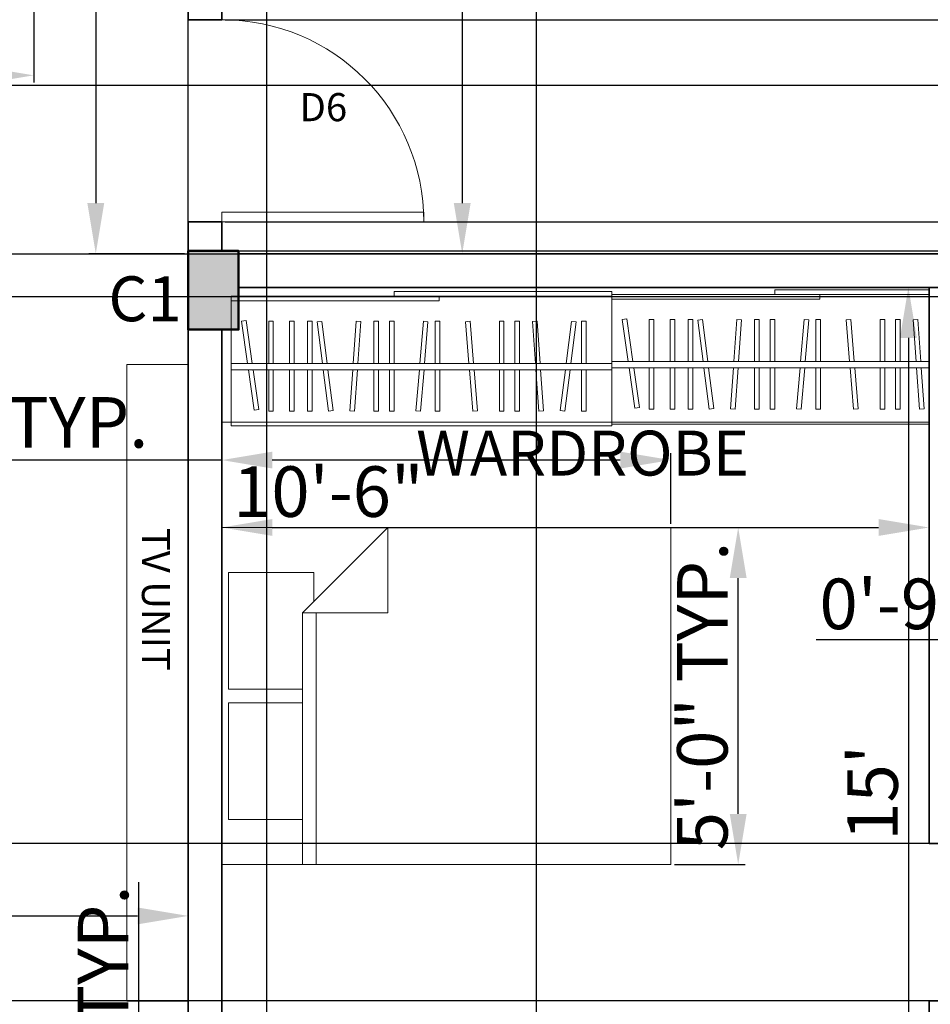
# Model space of a CAD drawing. Units: inches. Extents: x 2621 to 6190, y 513 to 1320.
# Tile 8 of 11: x 2997 to 3160, y 763 to 939. Entities that reach past the tile are written whole.
import ezdxf

# ---------------------------------------------------------------- set-up
doc = ezdxf.new("R2010")
doc.units = ezdxf.units.IN
for name, color, linetype, lineweight in [('A-ANNO-DIMS', 5, 'Continuous', 18), ('A-ANNO-TEXT', 7, 'Continuous', 18), ('A-FLOR-CASE', 30, 'Continuous', 18), ('A-WALL', 7, 'Continuous', 35), ('columns', 2, 'Continuous', 50), ('door', 1, 'Continuous', 18), ('furniture', 30, 'Continuous', 18), ('S-COLS-IDEN', 2, 'Continuous', 25), ('S-COLS-PATT', 2, 'Continuous', 13)]:
    doc.layers.add(name, color=color, linetype=linetype, lineweight=lineweight)
doc.styles.get("Standard").update_dxf_attribs({"font": 'arial.ttf'})
doc.dimstyles.new('ISO-25', dxfattribs={"dimtxt": 9, "dimasz": 9, "dimexe": 1.25, "dimexo": 0.625, "dimtad": 1, "dimlunit": 3, "dimtxsty": 'Standard', "dimcen": 2.5, "dimadec": 0, "dimazin": 0, "dimtfac": 1, "dimtmove": 0, "dimatfit": 3, "dimfxl": 1, "dimarcsym": 0})

# ---------------------------------------------------------------- blocks, each defined once
blk = doc.blocks.new('*U3')
for p, q in [((-28, 0), (-28, 6)), ((0, 0), (0, 6))]:
    blk.add_line(p, q)
blk.add_lwpolyline([(0, 0), (0, -28), (-1.75, -28), (-1.75, 0)], close=True)
blk.add_arc((0, 0), 28, 180, 270)
blk = doc.blocks.new('*U6')
for p, q in [((0, 0), (0, -6)), ((36, 0), (36, -6))]:
    blk.add_line(p, q)
blk.add_lwpolyline([(0, 0), (0, 36), (1.75, 36), (1.75, 0)], close=True)
blk.add_arc((0, 0), 36, 0, 90)
blk = doc.blocks.new('Bed - Queen')
for p, q in [((0, -80.00003), (0, 0)), ((0, 0), (59.99999, 0)), ((59.99999, 0), (59.99999, -80.00003)), ((7.99999, -1.2), (28.79998, -1.2)), ((7.99999, -14.4), (7.99999, -1.2)), ((28.79998, -1.2), (28.79998, -14.4)), ((31.19999, -1.2), (51.99999, -1.2)), ((31.19999, -14.4), (31.19999, -1.2)), ((51.99999, -1.2), (51.99999, -16.4)), ((0, -14.4), (44.8, -14.4)), ((59.99999, -29.6), (44.8, -14.4)), ((44.8, -14.4), (44.8, -29.6)), ((44.8, -16.8), (0, -16.8)), ((51.99999, -16.4), (46.79936, -16.4)), ((44.8, -29.6), (59.99999, -29.6)), ((59.99999, -80.00003), (0, -80.00003))]:
    blk.add_line(p, q)
blk = doc.blocks.new('*D22')
at = {"layer": 'A-ANNO-DIMS', "color": 0, "lineweight": -2, "transparency": 16777216}
for p, q in [((3026.76, 1076.89), (3009.69, 1076.89)), ((3010.94, 1067.89), (3010.94, 905.89)), ((3026.76, 896.89), (3009.69, 896.89))]:
    blk.add_line(p, q, dxfattribs=at)
at = {"layer": 'A-ANNO-DIMS', "color": 0, "transparency": 16777216}
for points in [[(3009.44, 1067.89), (3012.44, 1067.89), (3010.94, 1076.89)], [(3009.44, 905.89), (3012.44, 905.89), (3010.94, 896.89)]]:
    blk.add_solid(points, dxfattribs=at)
at = {"layer": 'Defpoints', "color": 0, "transparency": 16777216}
for p in [(3027.38, 1076.89), (3010.94, 896.89), (3027.38, 896.89)]:
    blk.add_point(p, dxfattribs=at)
at = {"layer": 'A-ANNO-DIMS', "color": 0, "transparency": 16777216, "insert": (3005.72, 986.89), "char_height": 9, "attachment_point": 5, "rotation": 90}
blk.add_mtext("15'", dxfattribs=at)
blk = doc.blocks.new('*D23')
at = {"layer": 'A-ANNO-DIMS', "color": 0, "lineweight": -2, "transparency": 16777216}
for p, q in [((3069.48, 1076.89), (3077.47, 1076.89)), ((3076.22, 1067.89), (3076.22, 905.89)), ((3069.48, 896.89), (3077.47, 896.89))]:
    blk.add_line(p, q, dxfattribs=at)
at = {"layer": 'A-ANNO-DIMS', "color": 0, "transparency": 16777216}
for points in [[(3074.72, 1067.89), (3077.72, 1067.89), (3076.22, 1076.89)], [(3074.72, 905.89), (3077.72, 905.89), (3076.22, 896.89)]]:
    blk.add_solid(points, dxfattribs=at)
at = {"layer": 'Defpoints', "color": 0, "transparency": 16777216}
for p in [(3068.85, 1076.89), (3068.85, 896.89), (3076.22, 896.89)]:
    blk.add_point(p, dxfattribs=at)
at = {"layer": 'A-ANNO-DIMS', "color": 0, "transparency": 16777216, "insert": (3071, 986.89), "char_height": 9, "attachment_point": 5, "rotation": 90}
blk.add_mtext("15'", dxfattribs=at)
blk = doc.blocks.new('*D26')
at = {"layer": 'A-ANNO-DIMS', "color": 0, "lineweight": -2, "transparency": 16777216}
for p, q in [((2787.38, 779.61), (2787.38, 780.23)), ((3027.38, 779.61), (3027.38, 780.23)), ((2796.38, 778.98), (3018.38, 778.98))]:
    blk.add_line(p, q, dxfattribs=at)
at = {"layer": 'A-ANNO-DIMS', "color": 0, "transparency": 16777216}
for points in [[(2796.38, 780.48), (2796.38, 777.48), (2787.38, 778.98)], [(3018.38, 780.48), (3018.38, 777.48), (3027.38, 778.98)]]:
    blk.add_solid(points, dxfattribs=at)
at = {"layer": 'Defpoints', "color": 0, "transparency": 16777216}
for p in [(2787.38, 778.98), (3027.38, 778.98), (3027.38, 778.98)]:
    blk.add_point(p, dxfattribs=at)
at = {"layer": 'A-ANNO-DIMS', "color": 0, "transparency": 16777216, "insert": (2907.38, 784.21), "char_height": 9, "attachment_point": 5}
blk.add_mtext("20'", dxfattribs=at)
blk = doc.blocks.new('*D27')
at = {"layer": 'A-ANNO-DIMS', "color": 0, "lineweight": -2, "transparency": 16777216}
for p, q in [((3033.38, 851.83), (3033.38, 846.89)), ((3159.38, 851.83), (3159.38, 846.89)), ((3042.38, 848.14), (3150.38, 848.14))]:
    blk.add_line(p, q, dxfattribs=at)
at = {"layer": 'A-ANNO-DIMS', "color": 0, "transparency": 16777216}
for points in [[(3042.38, 849.64), (3042.38, 846.64), (3033.38, 848.14)], [(3150.38, 849.64), (3150.38, 846.64), (3159.38, 848.14)]]:
    blk.add_solid(points, dxfattribs=at)
at = {"layer": 'Defpoints', "color": 0, "transparency": 16777216}
for p in [(3033.38, 852.46), (3159.38, 852.46), (3159.38, 848.14)]:
    blk.add_point(p, dxfattribs=at)
at = {"layer": 'A-ANNO-DIMS', "color": 0, "transparency": 16777216, "insert": (3052.37, 853.36), "char_height": 9, "attachment_point": 5}
blk.add_mtext('10\'-6"', dxfattribs=at)
blk = doc.blocks.new('*D28')
at = {"layer": 'A-ANNO-DIMS', "color": 0, "lineweight": -2, "transparency": 16777216}
for p, q in [((3158.76, 890.89), (3154.45, 890.89)), ((3155.7, 881.89), (3155.7, 719.89)), ((3158.76, 710.89), (3154.45, 710.89))]:
    blk.add_line(p, q, dxfattribs=at)
at = {"layer": 'A-ANNO-DIMS', "color": 0, "transparency": 16777216}
for points in [[(3154.2, 881.89), (3157.2, 881.89), (3155.7, 890.89)], [(3154.2, 719.89), (3157.2, 719.89), (3155.7, 710.89)]]:
    blk.add_solid(points, dxfattribs=at)
at = {"layer": 'Defpoints', "color": 0, "transparency": 16777216}
for p in [(3159.38, 890.89), (3155.7, 710.89), (3159.38, 710.89)]:
    blk.add_point(p, dxfattribs=at)
at = {"layer": 'A-ANNO-DIMS', "color": 0, "transparency": 16777216, "insert": (3150.48, 800.89), "char_height": 9, "attachment_point": 5, "rotation": 90}
blk.add_mtext("15'", dxfattribs=at)
blk = doc.blocks.new('WARDROBE-HANGING-BAY')
for p, q in [((0, 0), (0, 67.83)), ((0, 67.83), (23.09, 67.83)), ((10.01, 67.78), (10.01, 0)), ((11.13, 0), (11.13, 67.78)), ((23.09, 0), (0, 0))]:
    blk.add_line(p, q)
for points in [[(23.09, 30.8), (23.09, 67.83), (22.26, 67.83), (22.26, 30.8)], [(23.91, 38.78), (23.91, 0), (23.09, 0), (23.09, 38.78)]]:
    blk.add_lwpolyline(points, close=True)
for points in [[(11.13, 64.11), (18.75, 65.19), (18.63, 66.01), (11.13, 64.94)], [(10.01, 64.78), (2.81, 63.75), (2.92, 62.93)], [(2.92, 62.93), (10.01, 63.95)], [(10.01, 61.16), (2.65, 61.16), (2.65, 60.34)], [(2.65, 60.34), (10.01, 60.34)], [(11.13, 60.34), (18.63, 60.34), (18.63, 61.16), (11.13, 61.16)], [(10.01, 57.44), (2.65, 57.44), (2.65, 56.61)], [(2.65, 56.61), (10.01, 56.61)], [(11.13, 56.61), (18.63, 56.61), (18.63, 57.44), (11.13, 57.44)], [(10.01, 54.27), (2.65, 54.27), (2.65, 53.44)], [(2.65, 53.44), (10.01, 53.44)], [(11.13, 53.44), (18.63, 53.44), (18.63, 54.27), (11.13, 54.27)], [(10.01, 51.44), (2.66, 50.5), (2.76, 49.68)], [(11.13, 50.74), (18.62, 51.69), (18.52, 52.51), (11.13, 51.58)], [(2.76, 49.68), (10.01, 50.6)], [(10.01, 46.18), (2.7, 46.71), (2.64, 45.89)], [(2.64, 45.89), (10.01, 45.35)], [(11.13, 45.27), (18.58, 44.73), (18.64, 45.56), (11.13, 46.1)], [(10.01, 42.41), (2.65, 42.41), (2.65, 41.58)], [(11.13, 41.58), (18.63, 41.58), (18.63, 42.41), (11.13, 42.41)], [(2.65, 41.58), (10.01, 41.58)], [(10.01, 39.65), (2.65, 39.65), (2.65, 38.83)], [(2.65, 38.83), (10.01, 38.83)], [(11.13, 38.83), (18.63, 38.83), (18.63, 39.65), (11.13, 39.65)], [(10.01, 34.32), (2.7, 34.93), (2.63, 34.1)], [(2.63, 34.1), (10.01, 33.49)], [(11.13, 33.39), (18.56, 32.78), (18.63, 33.6), (11.13, 34.22)], [(10.01, 31.52), (2.65, 31.52), (2.65, 30.69)], [(2.65, 30.69), (10.01, 30.69)], [(11.13, 30.69), (18.63, 30.69), (18.63, 31.52), (11.13, 31.52)], [(2.63, 24.79), (10.01, 25.4)], [(10.01, 24.57), (2.7, 23.96), (2.63, 24.79)], [(11.13, 25.5), (18.56, 26.12), (18.63, 25.29), (11.13, 24.67)], [(2.65, 20.07), (10.01, 20.07)], [(10.01, 19.24), (2.65, 19.24), (2.65, 20.07)], [(11.13, 20.07), (18.63, 20.07), (18.63, 19.24), (11.13, 19.24)], [(10.01, 16.48), (2.65, 16.48), (2.65, 17.31)], [(2.65, 17.31), (10.01, 17.31)], [(11.13, 17.31), (18.63, 17.31), (18.63, 16.48), (11.13, 16.48)], [(11.13, 13.62), (18.58, 14.16), (18.64, 13.34), (11.13, 12.79)], [(2.64, 13.01), (10.01, 13.54)], [(10.01, 12.71), (2.7, 12.18), (2.64, 13.01)], [(10.01, 7.46), (2.66, 8.39), (2.76, 9.21)], [(2.76, 9.21), (10.01, 8.29)], [(11.13, 8.15), (18.62, 7.2), (18.52, 6.38), (11.13, 7.31)], [(10.01, 4.62), (2.65, 4.62), (2.65, 5.45)], [(2.65, 5.45), (10.01, 5.45)], [(11.13, 5.45), (18.63, 5.45), (18.63, 4.62), (11.13, 4.62)]]:
    blk.add_lwpolyline(points)
blk = doc.blocks.new('*D54')
at = {"layer": 'A-ANNO-DIMS', "color": 0, "lineweight": -2, "transparency": 16777216}
for p, q in [((3018.62, 719.89), (3018.62, 785)), ((3020.69, 710.89), (3017.37, 710.89)), ((3018.62, 701.89), (3018.62, 710.89)), ((3020.69, 701.89), (3017.37, 701.89)), ((3018.62, 692.89), (3018.62, 683.89))]:
    blk.add_line(p, q, dxfattribs=at)
at = {"layer": 'A-ANNO-DIMS', "color": 0, "transparency": 16777216}
for points in [[(3017.12, 719.89), (3020.12, 719.89), (3018.62, 710.89)], [(3017.12, 692.89), (3020.12, 692.89), (3018.62, 701.89)]]:
    blk.add_solid(points, dxfattribs=at)
at = {"layer": 'Defpoints', "color": 0, "transparency": 16777216}
for p in [(3018.62, 710.89), (3021.32, 710.89), (3021.32, 701.89)]:
    blk.add_point(p, dxfattribs=at)
at = {"layer": 'A-ANNO-DIMS', "color": 0, "transparency": 16777216, "insert": (3013.4, 756.94), "char_height": 9, "attachment_point": 5, "rotation": 90}
blk.add_mtext('0\'-9" TYP.', dxfattribs=at)
blk = doc.blocks.new('*D58')
at = {"layer": 'A-ANNO-DIMS', "color": 0, "lineweight": -2, "transparency": 16777216}
for p, q in [((3213.38, 831.12), (3213.38, 826.89)), ((3222.38, 831.12), (3222.38, 826.89)), ((3204.38, 828.14), (3139.27, 828.14)), ((3222.38, 828.14), (3213.38, 828.14)), ((3231.38, 828.14), (3240.38, 828.14))]:
    blk.add_line(p, q, dxfattribs=at)
at = {"layer": 'A-ANNO-DIMS', "color": 0, "transparency": 16777216}
for points in [[(3204.38, 829.64), (3204.38, 826.64), (3213.38, 828.14)], [(3231.38, 829.64), (3231.38, 826.64), (3222.38, 828.14)]]:
    blk.add_solid(points, dxfattribs=at)
at = {"layer": 'Defpoints', "color": 0, "transparency": 16777216}
for p in [(3213.38, 831.74), (3222.38, 831.74), (3213.38, 828.14)]:
    blk.add_point(p, dxfattribs=at)
at = {"layer": 'A-ANNO-DIMS', "color": 0, "transparency": 16777216, "insert": (3167.33, 833.37), "char_height": 9, "attachment_point": 5}
blk.add_mtext('0\'-9" TYP.', dxfattribs=at)
blk = doc.blocks.new('*D63')
at = {"layer": 'A-ANNO-DIMS', "color": 0, "lineweight": -2, "transparency": 16777216}
for p, q in [((3033.38, 848.76), (3033.38, 861.39)), ((3113.38, 848.76), (3113.38, 861.39)), ((3033.38, 860.14), (2890.74, 860.14)), ((3104.38, 860.14), (3042.38, 860.14))]:
    blk.add_line(p, q, dxfattribs=at)
at = {"layer": 'A-ANNO-DIMS', "color": 0, "transparency": 16777216}
for points in [[(3042.38, 861.64), (3042.38, 858.64), (3033.38, 860.14)], [(3104.38, 861.64), (3104.38, 858.64), (3113.38, 860.14)]]:
    blk.add_solid(points, dxfattribs=at)
at = {"layer": 'Defpoints', "color": 0, "transparency": 16777216}
for p in [(3033.38, 860.14), (3033.38, 848.14), (3113.38, 848.14)]:
    blk.add_point(p, dxfattribs=at)
at = {"layer": 'A-ANNO-DIMS', "color": 0, "transparency": 16777216, "insert": (2957.56, 865.69), "char_height": 9, "attachment_point": 5}
blk.add_mtext('QUEEN BED 6\'-8" TYP.', dxfattribs=at)
blk = doc.blocks.new('*D64')
at = {"layer": 'A-ANNO-DIMS', "color": 0, "lineweight": -2, "transparency": 16777216}
for p, q in [((3114.01, 848.14), (3126.63, 848.14)), ((3125.38, 797.14), (3125.38, 839.14)), ((3114.01, 788.14), (3126.63, 788.14))]:
    blk.add_line(p, q, dxfattribs=at)
at = {"layer": 'A-ANNO-DIMS', "color": 0, "transparency": 16777216}
for points in [[(3123.88, 839.14), (3126.88, 839.14), (3125.38, 848.14)], [(3123.88, 797.14), (3126.88, 797.14), (3125.38, 788.14)]]:
    blk.add_solid(points, dxfattribs=at)
at = {"layer": 'Defpoints', "color": 0, "transparency": 16777216}
for p in [(3113.38, 848.14), (3125.38, 848.14), (3113.38, 788.14)]:
    blk.add_point(p, dxfattribs=at)
at = {"layer": 'A-ANNO-DIMS', "color": 0, "transparency": 16777216, "insert": (3120.16, 818.14), "char_height": 9, "attachment_point": 5, "rotation": 90}
blk.add_mtext('5\'-0" TYP.', dxfattribs=at)
blk = doc.blocks.new('*D74')
at = {"layer": 'A-ANNO-DIMS', "color": 0, "lineweight": -2, "transparency": 16777216}
for p, q in [((2944.88, 941.67), (2944.88, 927.39)), ((2999.88, 941.67), (2999.88, 927.39)), ((2953.88, 928.64), (2990.88, 928.64))]:
    blk.add_line(p, q, dxfattribs=at)
at = {"layer": 'A-ANNO-DIMS', "color": 0, "transparency": 16777216}
for points in [[(2953.88, 930.14), (2953.88, 927.14), (2944.88, 928.64)], [(2990.88, 930.14), (2990.88, 927.14), (2999.88, 928.64)]]:
    blk.add_solid(points, dxfattribs=at)
at = {"layer": 'Defpoints', "color": 0, "transparency": 16777216}
for p in [(2944.88, 942.29), (2999.88, 942.29), (2999.88, 928.64)]:
    blk.add_point(p, dxfattribs=at)
at = {"layer": 'A-ANNO-DIMS', "color": 0, "transparency": 16777216, "insert": (2972.38, 933.77), "char_height": 9, "attachment_point": 5}
blk.add_mtext('4\'-7"', dxfattribs=at)
blk = doc.blocks.new('*D82')
at = {"layer": 'A-ANNO-DIMS', "color": 0, "lineweight": -2, "transparency": 16777216}
for p, q in [((2924.85, 889.24), (3291.63, 889.24)), ((3290.38, 719.89), (3290.38, 880.24)), ((2917.49, 710.89), (3291.63, 710.89))]:
    blk.add_line(p, q, dxfattribs=at)
at = {"layer": 'A-ANNO-DIMS', "color": 0, "transparency": 16777216}
for points in [[(3288.88, 880.24), (3291.88, 880.24), (3290.38, 889.24)], [(3288.88, 719.89), (3291.88, 719.89), (3290.38, 710.89)]]:
    blk.add_solid(points, dxfattribs=at)
at = {"layer": 'Defpoints', "color": 0, "transparency": 16777216}
for p in [(2924.22, 889.24), (3290.38, 889.24), (2916.87, 710.89)]:
    blk.add_point(p, dxfattribs=at)
at = {"layer": 'A-ANNO-DIMS', "color": 0, "transparency": 16777216, "insert": (3285.1, 800.07), "char_height": 9, "attachment_point": 5, "rotation": 90}
blk.add_mtext('14\'-10 1/2"', dxfattribs=at)
blk = doc.blocks.new('*D83')
at = {"layer": 'A-ANNO-DIMS', "color": 0, "lineweight": -2, "transparency": 16777216}
for p, q in [((3028.01, 1085.89), (3291.63, 1085.89)), ((3290.38, 906.39), (3290.38, 1076.89)), ((3028.01, 897.39), (3291.63, 897.39))]:
    blk.add_line(p, q, dxfattribs=at)
at = {"layer": 'A-ANNO-DIMS', "color": 0, "transparency": 16777216}
for points in [[(3288.88, 1076.89), (3291.88, 1076.89), (3290.38, 1085.89)], [(3288.88, 906.39), (3291.88, 906.39), (3290.38, 897.39)]]:
    blk.add_solid(points, dxfattribs=at)
at = {"layer": 'Defpoints', "color": 0, "transparency": 16777216}
for p in [(3027.38, 1085.89), (3290.38, 1085.89), (3027.38, 897.39)]:
    blk.add_point(p, dxfattribs=at)
at = {"layer": 'A-ANNO-DIMS', "color": 0, "transparency": 16777216, "insert": (3285.1, 991.64), "char_height": 9, "attachment_point": 5, "rotation": 90}
blk.add_mtext('15\'-8 1/2"', dxfattribs=at)
blk = doc.blocks.new('*D88')
at = {"layer": 'A-ANNO-DIMS', "color": 0, "lineweight": -2, "transparency": 16777216}
for p, q in [((2910.22, 898.87), (2910.22, 1155.14)), ((2919.22, 1153.89), (3018.38, 1153.89)), ((3027.38, 898.01), (3027.38, 1155.14))]:
    blk.add_line(p, q, dxfattribs=at)
at = {"layer": 'A-ANNO-DIMS', "color": 0, "transparency": 16777216}
for points in [[(2919.22, 1155.39), (2919.22, 1152.39), (2910.22, 1153.89)], [(3018.38, 1155.39), (3018.38, 1152.39), (3027.38, 1153.89)]]:
    blk.add_solid(points, dxfattribs=at)
at = {"layer": 'Defpoints', "color": 0, "transparency": 16777216}
for p in [(3027.38, 1153.89), (2910.22, 898.24), (3027.38, 897.39)]:
    blk.add_point(p, dxfattribs=at)
at = {"layer": 'A-ANNO-DIMS', "color": 0, "transparency": 16777216, "insert": (2968.8, 1159.11), "char_height": 9, "attachment_point": 5}
blk.add_mtext('9\'-9"', dxfattribs=at)
blk = doc.blocks.new('*D97')
at = {"layer": 'A-ANNO-DIMS', "color": 0, "lineweight": -2, "transparency": 16777216}
for p, q in [((3164.76, 791.89), (2685.13, 791.89)), ((2686.38, 772.89), (2686.38, 782.89)), ((3164.76, 763.89), (2685.13, 763.89))]:
    blk.add_line(p, q, dxfattribs=at)
at = {"layer": 'A-ANNO-DIMS', "color": 0, "transparency": 16777216}
for points in [[(2684.88, 782.89), (2687.88, 782.89), (2686.38, 791.89)], [(2684.88, 772.89), (2687.88, 772.89), (2686.38, 763.89)]]:
    blk.add_solid(points, dxfattribs=at)
at = {"layer": 'Defpoints', "color": 0, "transparency": 16777216}
for p in [(2686.38, 791.89), (3165.38, 791.89), (3165.38, 763.89)]:
    blk.add_point(p, dxfattribs=at)
at = {"layer": 'A-ANNO-DIMS', "color": 0, "transparency": 16777216, "insert": (2681.24, 777.89), "char_height": 9, "attachment_point": 5, "rotation": 90}
blk.add_mtext('2\'-4"', dxfattribs=at)
blk = doc.blocks.new('*D99')
at = {"layer": 'A-ANNO-DIMS', "color": 0, "lineweight": -2, "transparency": 16777216}
for p, q in [((3034.01, 938.55), (3291.63, 938.55)), ((3290.38, 911.55), (3290.38, 929.55)), ((3034.01, 902.55), (3291.63, 902.55))]:
    blk.add_line(p, q, dxfattribs=at)
at = {"layer": 'A-ANNO-DIMS', "color": 0, "transparency": 16777216}
for points in [[(3288.88, 929.55), (3291.88, 929.55), (3290.38, 938.55)], [(3288.88, 911.55), (3291.88, 911.55), (3290.38, 902.55)]]:
    blk.add_solid(points, dxfattribs=at)
at = {"layer": 'Defpoints', "color": 0, "transparency": 16777216}
for p in [(3033.38, 938.55), (3290.38, 938.55), (3033.38, 902.55)]:
    blk.add_point(p, dxfattribs=at)
at = {"layer": 'A-ANNO-DIMS', "color": 0, "transparency": 16777216, "insert": (3285.16, 920.55), "char_height": 9, "attachment_point": 5, "rotation": 90}
blk.add_mtext('3\'-0"', dxfattribs=at)
blk = doc.blocks.new('*D100')
at = {"layer": 'A-ANNO-DIMS', "color": 0, "lineweight": -2, "transparency": 16777216}
for p, q in [((2854.01, 926.89), (3291.63, 926.89)), ((3290.38, 905.89), (3290.38, 917.89)), ((2854.01, 896.89), (3291.63, 896.89))]:
    blk.add_line(p, q, dxfattribs=at)
at = {"layer": 'A-ANNO-DIMS', "color": 0, "transparency": 16777216}
for points in [[(3288.88, 917.89), (3291.88, 917.89), (3290.38, 926.89)], [(3288.88, 905.89), (3291.88, 905.89), (3290.38, 896.89)]]:
    blk.add_solid(points, dxfattribs=at)
at = {"layer": 'Defpoints', "color": 0, "transparency": 16777216}
for p in [(2853.38, 926.89), (3290.38, 926.89), (2853.38, 896.89)]:
    blk.add_point(p, dxfattribs=at)
at = {"layer": 'A-ANNO-DIMS', "color": 0, "transparency": 16777216, "insert": (3285.16, 911.89), "char_height": 9, "attachment_point": 5, "rotation": 90}
blk.add_mtext('2\'-6"', dxfattribs=at)
blk = doc.blocks.new('*D102')
at = {"layer": 'A-ANNO-DIMS', "color": 0, "lineweight": -2, "transparency": 16777216}
for p, q in [((2915.57, 1054.4), (2915.57, 519.64)), ((2942.88, 1054.4), (2942.88, 519.64)), ((2924.57, 520.89), (2933.88, 520.89)), ((2942.88, 520.89), (2998.18, 520.89))]:
    blk.add_line(p, q, dxfattribs=at)
at = {"layer": 'A-ANNO-DIMS', "color": 0, "transparency": 16777216}
for points in [[(2924.57, 522.39), (2924.57, 519.39), (2915.57, 520.89)], [(2933.88, 522.39), (2933.88, 519.39), (2942.88, 520.89)]]:
    blk.add_solid(points, dxfattribs=at)
at = {"layer": 'Defpoints', "color": 0, "transparency": 16777216}
for p in [(2915.57, 1055.03), (2942.88, 1055.03), (2942.88, 520.89)]:
    blk.add_point(p, dxfattribs=at)
at = {"layer": 'A-ANNO-DIMS', "color": 0, "transparency": 16777216, "insert": (2975.03, 526.17), "char_height": 9, "attachment_point": 5}
blk.add_mtext('2\'-3 1/2"', dxfattribs=at)
blk = doc.blocks.new('*D107')
at = {"layer": 'A-ANNO-DIMS', "color": 0, "lineweight": -2, "transparency": 16777216}
for p, q in [((3041.38, 1076.26), (3041.38, 519.64)), ((3089.38, 1076.26), (3089.38, 519.64)), ((3050.38, 520.89), (3080.38, 520.89))]:
    blk.add_line(p, q, dxfattribs=at)
at = {"layer": 'A-ANNO-DIMS', "color": 0, "transparency": 16777216}
for points in [[(3050.38, 522.39), (3050.38, 519.39), (3041.38, 520.89)], [(3080.38, 522.39), (3080.38, 519.39), (3089.38, 520.89)]]:
    blk.add_solid(points, dxfattribs=at)
at = {"layer": 'Defpoints', "color": 0, "transparency": 16777216}
for p in [(3041.38, 1076.89), (3089.38, 1076.89), (3089.38, 520.89)]:
    blk.add_point(p, dxfattribs=at)
at = {"layer": 'A-ANNO-DIMS', "color": 0, "transparency": 16777216, "insert": (3065.38, 526.11), "char_height": 9, "attachment_point": 5}
blk.add_mtext('4\'-0"', dxfattribs=at)

msp = doc.modelspace()

# ---------------------------------------------------------------- hatches: boundary and pattern name
at = {"layer": 'S-COLS-PATT'}
h = msp.add_hatch(color=256, dxfattribs=at)
h.dxf.hatch_style = 1
h.paths.add_polyline_path([(2787.381, 1085.89), (2778.381, 1085.89), (2778.381, 1071.89), (2787.381, 1071.89)])
h.paths.add_polyline_path([(3222.381, 1085.89), (3208.381, 1085.89), (3208.381, 1076.89), (3222.381, 1076.89)])
h.paths.add_polyline_path([(3041.381, 1085.89), (3027.381, 1085.89), (3027.381, 1076.89), (3041.381, 1076.89)])
h.paths.add_polyline_path([(2916.381, 1085.89), (2907.381, 1085.89), (2907.381, 1076.89), (2916.381, 1076.89)])
h.paths.add_polyline_path([(2916.381, 1076.89), (2913.381, 1076.89), (2913.381, 1071.89), (2916.381, 1071.89)])
h.paths.add_polyline_path([(2913.381, 1076.89), (2907.381, 1076.89), (2907.381, 1071.89), (2913.381, 1071.89)])
h.paths.add_polyline_path([(2787.381, 896.89), (2778.381, 896.89), (2778.381, 882.89), (2787.381, 882.89)])
h.paths.add_polyline_path([(2924.221, 898.241), (2910.221, 898.241), (2910.221, 889.241), (2924.221, 889.241)])
h.paths.add_polyline_path([(3036.381, 896.89), (3033.381, 896.89), (3027.381, 897.385), (3027.381, 883.385), (3033.381, 883.385), (3033.381, 890.89), (3036.381, 890.89)])
h.paths.add_polyline_path([(3036.381, 890.89), (3033.381, 890.89), (3033.381, 883.385), (3036.381, 883.385)], flags=17)
h.paths.add_polyline_path([(3222.381, 897.745), (3213.381, 897.745), (3213.381, 883.745), (3222.381, 883.745)])
h.paths.add_polyline_path([(3222.381, 710.89), (3208.381, 710.89), (3208.381, 701.89), (3222.381, 701.89)])
h.paths.add_polyline_path([(3039.318, 710.89), (3021.318, 710.89), (3021.318, 701.89), (3039.318, 701.89)])
h.paths.add_polyline_path([(2796.381, 710.89), (2778.381, 710.89), (2778.381, 701.89), (2796.381, 701.89)])
h = msp.add_hatch(color=256, dxfattribs=at)
h.dxf.hatch_style = 1
h.paths.add_polyline_path([(3036.381, 897.385), (3027.381, 897.385), (3027.381, 883.385), (3036.381, 883.385)])

# ---------------------------------------------------------------- linework, layer by layer
at = {"layer": 'A-FLOR-CASE'}
for p, q in [((3102.887, 866.554), (3102.887, 889.64)), ((3027.381, 877.163), (3016.458, 877.163)), ((3016.458, 877.163), (3016.458, 763.784)), ((3159.381, 877.687), (3102.929, 877.687)), ((3102.929, 876.563), (3159.381, 876.563)), ((3159.381, 866.89), (3033.381, 866.89)), ((3159.381, 866.554), (3102.887, 866.554)), ((3016.458, 763.784), (3027.381, 763.784))]:
    msp.add_line(p, q, dxfattribs=at)
msp.add_lwpolyline([(3139.915, 889.64), (3102.887, 889.64), (3102.887, 888.813), (3139.915, 888.813)], close=True, dxfattribs=at)
for points in [[(3159.381, 889.64), (3131.929, 889.64), (3131.929, 890.467), (3159.381, 890.467)], [(3106.606, 877.687), (3105.518, 885.304), (3104.699, 885.187), (3105.77, 877.687)], [(3110.375, 877.687), (3110.375, 885.188), (3109.548, 885.188), (3109.548, 877.687)], [(3114.098, 877.687), (3114.098, 885.188), (3113.271, 885.188), (3113.271, 877.687)], [(3117.27, 877.687), (3117.27, 885.188), (3116.442, 885.188), (3116.442, 877.687)], [(3119.968, 877.687), (3119.02, 885.176), (3118.199, 885.072), (3119.135, 877.687)], [(3125.442, 877.687), (3125.982, 885.137), (3125.157, 885.197), (3124.613, 877.687)], [(3129.128, 877.687), (3129.128, 885.188), (3128.301, 885.188), (3128.301, 877.687)], [(3131.886, 877.687), (3131.886, 885.188), (3131.059, 885.188), (3131.059, 877.687)], [(3137.318, 877.687), (3137.937, 885.114), (3137.112, 885.182), (3136.488, 877.687)], [(3140.022, 877.687), (3140.022, 885.188), (3139.194, 885.188), (3139.194, 877.687)], [(3145.215, 877.687), (3144.596, 885.114), (3145.421, 885.182), (3146.045, 877.687)], [(3150.647, 877.687), (3150.647, 885.188), (3151.474, 885.188), (3151.474, 877.687)], [(3153.405, 877.687), (3153.405, 885.188), (3154.232, 885.188), (3154.232, 877.687)], [(3157.091, 877.687), (3156.551, 885.137), (3157.377, 885.197), (3157.921, 877.687)], [(3105.931, 876.563), (3106.959, 869.36), (3107.778, 869.477)], [(3107.778, 869.477), (3106.766, 876.563)], [(3109.548, 876.563), (3109.548, 869.2), (3110.375, 869.2)], [(3110.375, 869.2), (3110.375, 876.563)], [(3113.271, 876.563), (3113.271, 869.2), (3114.098, 869.2)], [(3114.098, 869.2), (3114.098, 876.563)], [(3116.442, 876.563), (3116.442, 869.2), (3117.27, 869.2)], [(3117.27, 869.2), (3117.27, 876.563)], [(3119.277, 876.563), (3120.208, 869.212), (3121.029, 869.316)], [(3121.029, 869.316), (3120.111, 876.563)], [(3124.531, 876.563), (3124.002, 869.251), (3124.827, 869.191)], [(3124.827, 869.191), (3125.361, 876.563)], [(3128.301, 876.563), (3128.301, 869.2), (3129.128, 869.2)], [(3129.128, 869.2), (3129.128, 876.563)], [(3131.059, 876.563), (3131.059, 869.2), (3131.886, 869.2)], [(3131.886, 869.2), (3131.886, 876.563)], [(3136.395, 876.563), (3135.785, 869.25), (3136.61, 869.182)], [(3136.61, 869.182), (3137.225, 876.563)], [(3139.194, 876.563), (3139.194, 869.2), (3140.022, 869.2)], [(3140.022, 869.2), (3140.022, 876.563)], [(3145.923, 869.182), (3145.308, 876.563)], [(3146.139, 876.563), (3146.748, 869.25), (3145.923, 869.182)], [(3150.647, 869.2), (3150.647, 876.563)], [(3151.474, 876.563), (3151.474, 869.2), (3150.647, 869.2)], [(3154.232, 876.563), (3154.232, 869.2), (3153.405, 869.2)], [(3153.405, 869.2), (3153.405, 876.563)], [(3157.706, 869.191), (3157.172, 876.563)], [(3158.002, 876.563), (3158.532, 869.251), (3157.706, 869.191)]]:
    msp.add_lwpolyline(points, dxfattribs=at)
at = {"layer": 'A-WALL'}
for p, q in [((3027.381, 1076.89), (3027.381, 938.548)), ((3033.381, 1076.89), (3033.381, 938.548)), ((3027.381, 938.548), (3033.381, 938.548)), ((3027.381, 902.548), (3033.381, 902.548)), ((3027.381, 902.548), (3027.381, 752.89)), ((3033.381, 902.548), (3033.381, 897.385)), ((3171.381, 896.89), (3036.381, 896.89)), ((3171.381, 890.89), (3036.381, 890.89)), ((3159.381, 803.89), (3159.381, 890.89)), ((3033.381, 883.385), (3033.381, 752.89)), ((3159.381, 710.89), (3159.381, 763.89)), ((3159.381, 763.89), (3165.381, 763.89))]:
    msp.add_line(p, q, dxfattribs=at)
msp.add_lwpolyline([(3213.381, 797.89), (3199.381, 797.89), (3165.381, 797.89), (3165.381, 791.89), (3159.381, 791.89), (3159.381, 803.89)], dxfattribs=at)
at = {"layer": 'columns'}
msp.add_lwpolyline([(3027.381, 897.385), (3036.381, 897.385), (3036.381, 883.385), (3027.381, 883.385)], close=True, dxfattribs=at)

# ---------------------------------------------------------------- block references
at = {"layer": 'A-FLOR-CASE', "rotation": 89.99999999999991}
msp.add_blockref('WARDROBE-HANGING-BAY', (3102.899, 866.218), dxfattribs=at)
at = {"layer": 'door', "xscale": -1, "rotation": 270}
msp.add_blockref('*U6', (3033.381, 902.548), dxfattribs=at)
msp.add_blockref('*U6', (3033.381, 902.548), dxfattribs=at)
at = {"layer": 'door', "rotation": 90}
msp.add_blockref('*U3', (3165.381, 791.89), dxfattribs=at)
at = {"layer": 'furniture', "rotation": 90}
msp.add_blockref('Bed - Queen', (3033.381, 788.137), dxfattribs=at)

# ---------------------------------------------------------------- texts
at = {"layer": 'A-ANNO-TEXT', "attachment_point": 1}
for s, width, insert, char_height in [('D6', 12.30066, (3047.244, 925.477), 5), ('WARDROBE', 74.69403, (3068.012, 865.377), 8)]:
    msp.add_mtext_dynamic_manual_height_columns(s, width=width, gutter_width=12.5, heights=[0], dxfattribs=dict(at, insert=insert, char_height=char_height))
at = {"layer": 'A-ANNO-TEXT', "insert": (3024.163, 848.088), "char_height": 5, "attachment_point": 1, "rotation": 270}
msp.add_mtext_dynamic_manual_height_columns('TV UNIT  ', width=41.95014, gutter_width=12.5, heights=[0], dxfattribs=at)
at = {"layer": 'S-COLS-IDEN', "insert": (3013.191, 892.859), "char_height": 8, "attachment_point": 1}
msp.add_mtext_dynamic_manual_height_columns('C1', width=53.01391, gutter_width=12.5, heights=[0], dxfattribs=at)

# ---------------------------------------------------------------- dimensions: what is measured, and where the dimension line sits
at = {"layer": 'A-ANNO-DIMS'}
for base, p1, p2, override, picture, middle in [((3027.381, 1153.89), (2910.221, 898.241), (3027.381, 897.385), {"dimdec": 1, "dimlfac": 1, "dimrnd": 0, "dimzin": 1, "dimdsep": 46, "dimlunit": 4, "dimfrac": 2}, '*D88', (2968.801, 1159.11)), ((3089.381, 520.89), (3041.381, 1076.89), (3089.381, 1076.89), {"dimdec": 1, "dimlfac": 1, "dimrnd": 0, "dimzin": 1, "dimdsep": 46, "dimlunit": 4, "dimfrac": 2}, '*D107', (3065.381, 526.11)), ((2942.877, 520.89), (2915.573, 1055.025), (2942.877, 1055.025), {"dimdec": 1, "dimlfac": 1, "dimrnd": 0, "dimzin": 1, "dimdsep": 46, "dimlunit": 4, "dimfrac": 2}, '*D102', (2975.027, 526.171)), ((2999.881, 928.641), (2944.881, 942.291), (2999.881, 942.291), {"dimdec": 1, "dimlfac": 1, "dimrnd": 0, "dimzin": 1, "dimdsep": 46, "dimlunit": 4, "dimfrac": 2}, '*D74', (2972.381, 933.766)), ((3027.381, 778.985), (2787.381, 778.985), (3027.381, 778.985), {"dimclrd": 0, "dimclre": 0, "dimclrt": 0}, '*D26', (2907.381, 784.205))]:
    dim = msp.add_linear_dim(base=base, p1=p1, p2=p2, dimstyle='ISO-25', override=override, dxfattribs=at)
    dim.commit()
    dim.dimension.update_dxf_attribs({"geometry": picture, "text_midpoint": middle})
for base, p1, p2, override, picture, middle in [((3290.381, 1085.89), (3027.381, 897.385), (3027.381, 1085.89), {"dimdec": 1, "dimlfac": 1, "dimrnd": 0, "dimzin": 1, "dimdsep": 46, "dimlunit": 4, "dimfrac": 2}, '*D83', (3285.103, 991.637)), ((3010.942, 896.89), (3027.381, 1076.89), (3027.381, 896.89), {"dimclrd": 0, "dimclre": 0, "dimclrt": 0}, '*D22', (3005.722, 986.89)), ((3076.22, 896.89), (3068.85, 1076.89), (3068.85, 896.89), {"dimclrd": 0, "dimclre": 0, "dimclrt": 0}, '*D23', (3071, 986.89)), ((3290.381, 938.548), (3033.381, 902.548), (3033.381, 938.548), {"dimdec": 1, "dimlfac": 1, "dimrnd": 0, "dimzin": 1, "dimdsep": 46, "dimlunit": 4, "dimfrac": 2}, '*D99', (3285.158, 920.548)), ((3290.381, 926.89), (2853.381, 896.89), (2853.381, 926.89), {"dimdec": 1, "dimlfac": 1, "dimrnd": 0, "dimzin": 1, "dimdsep": 46, "dimlunit": 4, "dimfrac": 2}, '*D100', (3285.161, 911.89)), ((3155.695, 710.89), (3159.381, 890.89), (3159.381, 710.89), {"dimclrd": 0, "dimclre": 0, "dimclrt": 0}, '*D28', (3150.475, 800.89)), ((3290.381, 889.241), (2916.869, 710.89), (2924.221, 889.241), {"dimdec": 1, "dimlfac": 1, "dimrnd": 0, "dimzin": 1, "dimdsep": 46, "dimlunit": 4, "dimfrac": 2}, '*D82', (3285.103, 800.065)), ((2686.381, 791.89), (3165.381, 763.89), (3165.381, 791.89), {"dimdec": 1, "dimlfac": 1, "dimrnd": 0, "dimzin": 1, "dimdsep": 46, "dimlunit": 4, "dimfrac": 2}, '*D97', (2681.238, 777.89))]:
    dim = msp.add_linear_dim(base=base, p1=p1, p2=p2, angle=90, dimstyle='ISO-25', override=override, dxfattribs=at)
    dim.commit()
    dim.dimension.update_dxf_attribs({"geometry": picture, "text_midpoint": middle})
for base, p1, p2, angle, text, picture, middle in [((3033.381, 860.137), (3113.381, 848.137), (3033.381, 848.137), 180, 'QUEEN BED <> TYP.', '*D63', (2957.561, 865.692)), ((3125.381, 848.137), (3113.381, 788.137), (3113.381, 848.137), 90, '<> TYP.', '*D64', (3120.161, 818.137)), ((3213.381, 828.145), (3222.381, 831.745), (3213.381, 831.745), 180, '<> TYP.', '*D58', (3167.326, 833.365)), ((3018.618, 710.89), (3021.318, 701.89), (3021.318, 710.89), 90, '<> TYP.', '*D54', (3013.398, 756.944))]:
    dim = msp.add_linear_dim(base=base, p1=p1, p2=p2, angle=angle, text=text, dimstyle='ISO-25', override={"dimdec": 1, "dimlfac": 1, "dimrnd": 0, "dimzin": 1, "dimdsep": 46, "dimlunit": 4, "dimfrac": 2}, dxfattribs=at)
    dim.commit()
    dim.dimension.update_dxf_attribs({"geometry": picture, "text_midpoint": middle})
dim = msp.add_linear_dim(base=(3159.381, 848.137), p1=(3033.381, 852.459), p2=(3159.381, 852.459), dimstyle='ISO-25', override={"dimclrd": 0, "dimclre": 0, "dimclrt": 0}, dxfattribs=at)
dim.commit()
dim.dimension.update_dxf_attribs({"geometry": '*D27', "text_midpoint": (3052.368, 848.137), "dimtype": 160})

doc.saveas('drawing.dxf')
